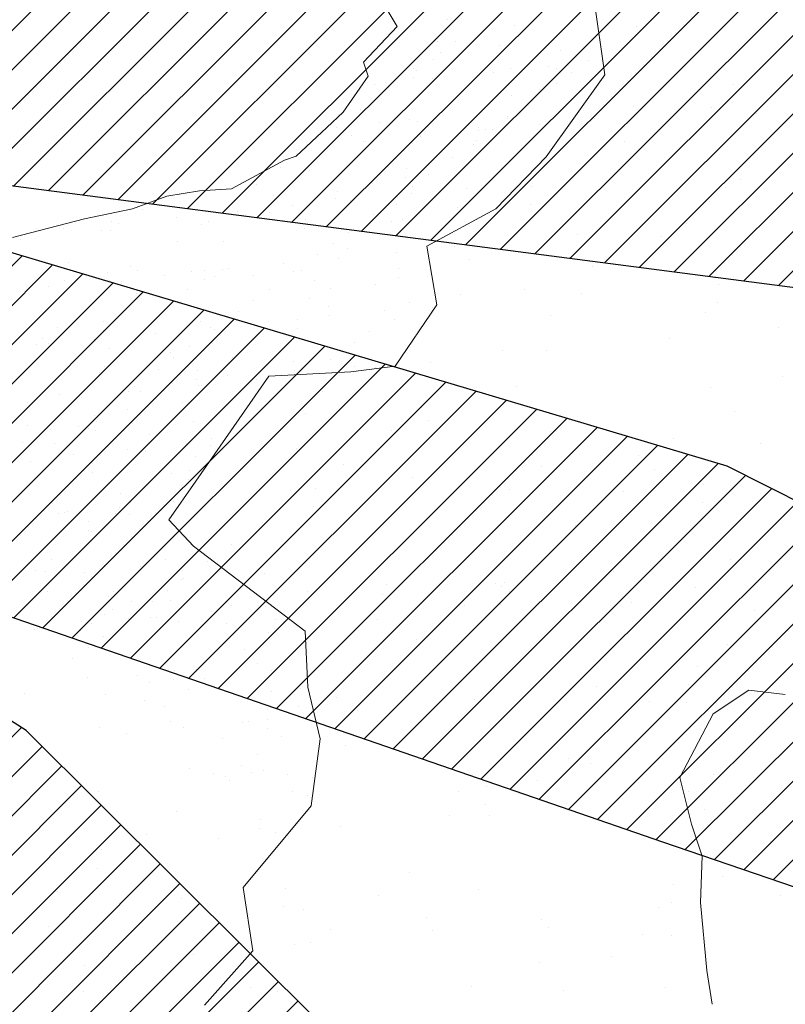
# Model space of a CAD drawing. Units: inches. Extents: x 1986 to 21484, y -1816 to 2016.
# Tile 69 of 85: x 3674.872 to 3679.11, y 1877.893 to 1883.347. Entities that reach past the tile are written whole.
import ezdxf

# ---------------------------------------------------------------- set-up
doc = ezdxf.new("R2010")
doc.units = ezdxf.units.IN
doc.layers.add('L-PLNT', color=84, linetype='Continuous', lineweight=13)
doc.layers.add('vfolhas', color=114, linetype='Continuous', lineweight=5)
for name, color, linetype in [('vfolha', 72, 'Continuous'), ('vfolha2', 110, 'Continuous'), ('vfolhas2', 102, 'Continuous')]:
    doc.layers.add(name, color=color, linetype=linetype)
pattern_1 = [(45, (-2446.5133113, 50.986076), (-0.004419417382, 0.004419417382), [])]

# ---------------------------------------------------------------- blocks, each defined once
blk = doc.blocks.new('arbusto_PB_verde_grande')
at = {"layer": 'vfolha2'}
h = blk.add_hatch(dxfattribs=at)
h.set_pattern_fill('ANSI31', color=256, scale=0.05, style=0)
h.set_pattern_definition(pattern_1)
h.paths.add_polyline_path([(0.02944, 0.35651), (0.00028, 0.09048), (0.02625, -0.03934), (0.047, 0.06233), (0.06189, 0.09731), (0.09372, 0.26573), (0.09955, 0.43473), (0.08789, 0.61313), (0.0645, 0.72266), (0.04988, 0.6851), (0.0236, 0.51294)])
h.paths.add_polyline_path([(0.30106, 0.43789), (0.14225, 0.24871), (0.26685, 0.30022)])
h.paths.add_polyline_path([(0.37995, 0.22817), (0.23697, 0.15193), (0.18428, 0.09364), (0.11122, 0.04358), (0.02625, -0.03934), (0.28061, 0.04667), (0.36829, 0.07798), (0.46756, 0.11239), (0.61068, 0.19376), (0.71585, 0.27823), (0.55813, 0.25948)])
h.paths.add_polyline_path([(0.56101, -0.29441), (0.72752, -0.32573), (0.59024, -0.2412), (0.42962, -0.15982), (0.02625, -0.03934), (0.14922, -0.14107), (0.18838, -0.16604), (0.41501, -0.24435)])
h.paths.add_polyline_path([(-0.27429, -0.44776), (-0.30352, -0.72628), (-0.23923, -0.64175), (-0.15457, -0.45716), (0.02625, -0.03934), (-0.16328, -0.25376)])
h.paths.add_polyline_path([(-0.51963, -0.24744), (-0.67736, -0.32573), (-0.59558, -0.35072), (-0.40574, -0.32882), (-0.21007, -0.20995), (0.02625, -0.03934), (-0.14874, -0.06595), (-0.31518, -0.09101), (-0.41452, -0.15048)])
h.paths.add_polyline_path([(-0.52546, 0.25007), (-0.70947, 0.24698), (-0.51963, 0.1093), (-0.32979, 0.02167), (-0.07567, -0.0128), (-0.04234, -0.02148), (-0.35024, 0.1312)])
at = {"layer": 'vfolhas'}
h = blk.add_hatch(dxfattribs=at)
h.set_pattern_fill('ANSI31', color=256, scale=0.05, style=0)
h.set_pattern_definition(pattern_1)
h.paths.add_polyline_path([(-0.07279, 0.50669), (-0.18085, 0.65063), (-0.2334, 0.67253), (-0.20712, 0.53176), (-0.10785, 0.25007), (0.02625, -0.03934), (0.00028, 0.09048), (0.00816, 0.16241), (-0.04939, 0.29079)])
h.paths.add_polyline_path([(0.09902, 0.41929), (0.09372, 0.26573), (0.07906, 0.18814), (0.15506, 0.36901), (0.26606, 0.5505), (0.28356, 0.63504), (0.2485, 0.68819), (0.25145, 0.63504), (0.20178, 0.54426)])
h.paths.add_polyline_path([(0.12295, 0.24073), (0.047, 0.06233), (0.02625, -0.03934), (0.11122, 0.04358), (0.18428, 0.09364), (0.27478, 0.19376), (0.3215, 0.25323), (0.44129, 0.38467), (0.47634, 0.57866), (0.41789, 0.45347), (0.28939, 0.30954)])
h.paths.add_polyline_path([(0.58145, -0.03779), (0.70707, 0.01536), (0.78591, 0.04667), (0.74796, 0.06549), (0.62818, 0.08423), (0.52595, 0.09048), (0.39745, 0.04358), (0.02625, -0.03934), (0.25728, -0.03154), (0.43834, -0.0347)])
h.paths.add_polyline_path([(0.52022, -0.03647), (0.43834, -0.0347), (0.25728, -0.03154), (0.02625, -0.03934), (0.17964, -0.08515), (0.53768, -0.13167), (0.69541, -0.15357), (0.78591, -0.07852), (0.70413, -0.10042)])
h.paths.add_polyline_path([(0.27189, -0.21929), (0.14922, -0.14107), (0.02625, -0.03934), (0.15794, -0.31007), (0.29522, -0.42585), (0.41789, -0.49157), (0.56396, -0.56669), (0.5114, -0.48532), (0.39456, -0.34139)])
h.paths.add_polyline_path([(-0.05818, -0.47591), (-0.02312, -0.61984), (0.047, -0.80134), (0.08494, -0.59794), (0.07911, -0.4071), (0.03527, -0.25376), (0.02625, -0.03934), (-0.03773, -0.26001)])
h.paths.add_polyline_path([(-0.24218, 0.14054), (-0.11073, 0.06858), (0.02625, -0.03934), (-0.04235, 0.10871), (-0.21007, 0.23757), (-0.36485, 0.33145), (-0.47874, 0.40341), (-0.54303, 0.46288), (-0.49041, 0.33145), (-0.39408, 0.22192)])
at = {"layer": 'vfolha'}
for p, q in [((0.53768, -0.13167), (0.17964, -0.08515)), ((0.39456, -0.34139), (0.27189, -0.21929))]:
    blk.add_line(p, q, dxfattribs=at)
at = {"layer": 'vfolha2'}
for p, q in [((0.42962, -0.15982), (0.02625, -0.03934)), ((0.59024, -0.2412), (0.42962, -0.15982)), ((0.18838, -0.16604), (0.41501, -0.24435)), ((0.41501, -0.24435), (0.56101, -0.29441))]:
    blk.add_line(p, q, dxfattribs=at)
at = {"layer": 'vfolhas2'}
blk.add_line((0.27189, -0.21929), (0.14922, -0.14107), dxfattribs=at)
blk = doc.blocks.new('PLANT-SHRUB')
for p, q in [((2160.9334, 1900.8779), (2161.0374, 1901.0337)), ((2160.3523, 1900.855), (2160.3523, 1900.855)), ((2160.6996, 1900.5794), (2160.9334, 1900.8779)), ((2161.1627, 1900.7886), (2161.1627, 1900.7886)), ((2160.1875, 1900.5998), (2160.1875, 1900.5998)), ((2160.5177, 1900.3976), (2160.6996, 1900.5794)), ((2160.6996, 1900.5794), (2160.6996, 1900.5794)), ((2160.9394, 1900.6033), (2160.9394, 1900.6033)), ((2160.5124, 1900.557), (2160.5124, 1900.557)), ((2160.815, 1900.47), (2160.815, 1900.47)), ((2161.0553, 1900.4856), (2161.0553, 1900.4856)), ((2160.8913, 1900.4413), (2160.8913, 1900.4413)), ((2161.2633, 1900.4582), (2161.2633, 1900.4582)), ((2161.5883, 1900.4154), (2161.5883, 1900.4154)), ((2160.4398, 1900.2289), (2160.5177, 1900.3976)), ((2160.7413, 1900.4025), (2160.7413, 1900.4025)), ((2160.3099, 1899.9952), (2160.4398, 1900.2289)), ((2160.3327, 1900.2167), (2160.3327, 1900.2167)), ((2161.5773, 1900.2145), (2161.5773, 1900.2145)), ((2160.1641, 1900.1094), (2160.1641, 1900.1094)), ((2160.3271, 1900.0849), (2160.3271, 1900.0849)), ((2161.4088, 1900.1071), (2161.4088, 1900.1071)), ((2159.5694, 1900.0601), (2159.6993, 1899.9044)), ((2160.3435, 1900.038), (2160.3435, 1900.038)), ((2161.4066, 1900.046), (2161.4066, 1900.046)), ((2161.9428, 1900.0517), (2161.9428, 1900.0517)), ((2159.9332, 1899.8654), (2160.3099, 1899.9952)), ((2159.6993, 1899.9044), (2159.9332, 1899.8654)), ((2159.9958, 1899.7194), (2159.9958, 1899.7194)), ((2159.82, 1899.6846), (2159.82, 1899.6846)), ((2159.9222, 1899.6519), (2159.9222, 1899.6519)), ((2160.8662, 1899.6713), (2160.8662, 1899.6713)), ((2161.545, 1899.6872), (2161.545, 1899.6872)), ((2161.8885, 1899.6762), (2161.8885, 1899.6762)), ((2159.372, 1899.6047), (2159.372, 1899.6047)), ((2159.611, 1899.6409), (2159.611, 1899.6409)), ((2159.819, 1899.6135), (2159.819, 1899.6135)), ((2160.6166, 1899.6024), (2160.6166, 1899.6024)), ((2161.8613, 1899.6002), (2161.8613, 1899.6002)), ((2160.1439, 1899.5708), (2160.1439, 1899.5708)), ((2160.6868, 1899.4993), (2160.6868, 1899.4993)), ((2160.8948, 1899.4719), (2160.8948, 1899.4719)), ((2161.2198, 1899.4291), (2161.2198, 1899.4291)), ((2161.1973, 1899.3686), (2161.1973, 1899.3686)), ((2161.7626, 1899.3576), (2161.7626, 1899.3576)), ((2161.9707, 1899.3303), (2161.9707, 1899.3303)), ((2162.7465, 1899.3364), (2162.7465, 1899.3364)), ((2159.2795, 1899.3099), (2159.2795, 1899.3099)), ((2159.5244, 1899.2874), (2159.5244, 1899.2874)), ((2160.3019, 1899.3148), (2160.3019, 1899.3148)), ((2161.1236, 1899.3011), (2161.1236, 1899.3011)), ((2161.3814, 1899.2759), (2161.3814, 1899.2759)), ((2162.2956, 1899.2875), (2162.2956, 1899.2875)), ((2160.0099, 1899.2159), (2160.0099, 1899.2159)), ((2161.2545, 1899.2136), (2161.2545, 1899.2136)), ((2162.4276, 1899.2625), (2162.4276, 1899.2625)), ((2162.4991, 1899.2114), (2162.4991, 1899.2114)), ((2162.8385, 1899.216), (2162.8385, 1899.216)), ((2159.8413, 1899.1085), (2159.8413, 1899.1085)), ((2161.086, 1899.1063), (2161.086, 1899.1063)), ((2162.3306, 1899.104), (2162.3306, 1899.104)), ((2162.6895, 1899.0787), (2163.0906, 1899.1151)), ((2162.4889, 1898.7872), (2162.6895, 1899.0787)), ((2162.3988, 1899.0178), (2162.3988, 1899.0178)), ((2158.7153, 1898.9534), (2158.7153, 1898.9534)), ((2159.1767, 1898.9688), (2159.1767, 1898.9688)), ((2160.7258, 1898.9366), (2160.7258, 1898.9366)), ((2162.3251, 1898.9503), (2162.3251, 1898.9503)), ((2159.103, 1898.9013), (2159.103, 1898.9013)), ((2159.7948, 1898.9145), (2159.7948, 1898.9145)), ((2160.841, 1898.9012), (2160.841, 1898.9012)), ((2161.8634, 1898.9061), (2161.8634, 1898.9061)), ((2162.9428, 1898.8672), (2162.9428, 1898.8672)), ((2161.9054, 1898.7143), (2162.4889, 1898.7872)), ((2162.4889, 1898.7872), (2162.4889, 1898.7872)), ((2158.3747, 1898.7689), (2158.3747, 1898.7689)), ((2158.6996, 1898.7261), (2158.6996, 1898.7261)), ((2161.6137, 1898.4774), (2161.9054, 1898.7143)), ((2162.1495, 1898.6865), (2162.1495, 1898.6865)), ((2159.2425, 1898.6546), (2159.2425, 1898.6546)), ((2159.4505, 1898.6272), (2159.4505, 1898.6272)), ((2160.3781, 1898.618), (2160.3781, 1898.618)), ((2161.877, 1898.6584), (2161.877, 1898.6584)), ((2159.0492, 1898.6039), (2159.0492, 1898.6039)), ((2159.7754, 1898.5845), (2159.7754, 1898.5845)), ((2160.2938, 1898.6016), (2160.2938, 1898.6016)), ((2161.5385, 1898.5994), (2161.5385, 1898.5994)), ((2161.7927, 1898.6047), (2161.7927, 1898.6047)), ((2161.9273, 1898.5858), (2161.9273, 1898.5858)), ((2161.9273, 1898.5858), (2161.9273, 1898.5858)), ((2162.1613, 1898.575), (2162.1613, 1898.575)), ((2162.1981, 1898.6088), (2162.1981, 1898.6088)), ((2162.7831, 1898.5971), (2162.7831, 1898.5971)), ((2163.5266, 1898.5995), (2163.5266, 1898.5995)), ((2158.2082, 1898.5531), (2158.2082, 1898.5531)), ((2158.7052, 1898.5367), (2158.7052, 1898.5367)), ((2159.2544, 1898.5398), (2159.2544, 1898.5398)), ((2160.2768, 1898.5447), (2160.2768, 1898.5447)), ((2160.3044, 1898.5505), (2160.3044, 1898.5505)), ((2160.3183, 1898.513), (2160.3183, 1898.513)), ((2161.3562, 1898.5058), (2161.3562, 1898.5058)), ((2160.5263, 1898.4856), (2160.5263, 1898.4856)), ((2161.4678, 1898.2224), (2161.6137, 1898.4774)), ((2161.6137, 1898.4774), (2161.6137, 1898.4774)), ((2161.8793, 1898.4991), (2161.8793, 1898.4991)), ((2162.4024, 1898.4924), (2162.4024, 1898.4924)), ((2163.4248, 1898.4973), (2163.4248, 1898.4973)), ((2160.8513, 1898.4428), (2160.8513, 1898.4428)), ((2161.9624, 1898.3927), (2161.9624, 1898.3927)), ((2161.3941, 1898.3714), (2161.3941, 1898.3714)), ((2161.6022, 1898.344), (2161.6022, 1898.344)), ((2161.6022, 1898.344), (2161.6022, 1898.344)), ((2161.6022, 1898.344), (2161.6022, 1898.344)), ((2162.0189, 1898.3513), (2162.0189, 1898.3513)), ((2161.5972, 1898.3209), (2161.5972, 1898.3209)), ((2161.7646, 1898.3226), (2161.7646, 1898.3226)), ((2161.9271, 1898.3012), (2161.9271, 1898.3012)), ((2161.9271, 1898.3012), (2161.9271, 1898.3012)), ((2162.0361, 1898.2868), (2162.0361, 1898.2868)), ((2162.1369, 1898.3014), (2162.1369, 1898.3014)), ((2161.5796, 1898.2672), (2161.5796, 1898.2672)), ((2161.5796, 1898.2672), (2161.5796, 1898.2672)), ((2161.7885, 1898.2334), (2161.7885, 1898.2334)), ((2162.1401, 1898.2731), (2162.1401, 1898.2731)), ((2162.47, 1898.2297), (2162.47, 1898.2297)), ((2163.1287, 1898.235), (2163.1287, 1898.235)), ((2158.3575, 1898.2181), (2158.3575, 1898.2181)), ((2158.4425, 1898.2174), (2158.4425, 1898.2174)), ((2158.6902, 1898.1833), (2158.6902, 1898.1833)), ((2159.6871, 1898.2151), (2159.6871, 1898.2151)), ((2159.9066, 1898.186), (2159.9066, 1898.186)), ((2160.9317, 1898.2128), (2160.9317, 1898.2128)), ((2161.2673, 1897.9855), (2161.4678, 1898.2224)), ((2161.5059, 1898.1997), (2161.5059, 1898.1997)), ((2161.5059, 1898.1997), (2161.5059, 1898.1997)), ((2161.7517, 1898.1997), (2161.7517, 1898.1997)), ((2162.1764, 1898.2106), (2162.1764, 1898.2106)), ((2162.1764, 1898.2106), (2162.1764, 1898.2106)), ((2162.678, 1898.2023), (2162.678, 1898.2023)), ((2163.421, 1898.2083), (2163.421, 1898.2083)), ((2158.2838, 1898.1506), (2158.2838, 1898.1506)), ((2159.7696, 1898.1444), (2159.7696, 1898.1444)), ((2160.8158, 1898.1311), (2160.8158, 1898.1311)), ((2161.7156, 1898.158), (2161.7156, 1898.158)), ((2161.8382, 1898.136), (2161.8382, 1898.136)), ((2161.8382, 1898.136), (2161.8382, 1898.136)), ((2163.0029, 1898.1596), (2163.0029, 1898.1596)), ((2158.2739, 1898.11), (2158.2739, 1898.11)), ((2159.5186, 1898.1077), (2159.5186, 1898.1077)), ((2160.7632, 1898.1055), (2160.7632, 1898.1055)), ((2161.6313, 1898.1043), (2161.6313, 1898.1043)), ((2161.8667, 1898.1141), (2161.8667, 1898.1141)), ((2162.0078, 1898.1032), (2162.0078, 1898.1032)), ((2162.0078, 1898.1032), (2162.0078, 1898.1032)), ((2162.2536, 1898.1032), (2162.2536, 1898.1032)), ((2162.9177, 1898.0971), (2162.9177, 1898.0971)), ((2163.2525, 1898.1009), (2163.2525, 1898.1009)), ((2161.5528, 1898.0174), (2161.5528, 1898.0174)), ((2161.3949, 1897.2203), (2161.2673, 1897.9855)), ((2161.5846, 1897.9358), (2161.5846, 1897.9358)), ((2162.1244, 1897.9164), (2162.1244, 1897.9164)), ((2162.781, 1897.9164), (2162.781, 1897.9164)), ((2159.5589, 1897.8673), (2159.5589, 1897.8673)), ((2161.3139, 1897.8645), (2161.3139, 1897.8645)), ((2161.379, 1897.8581), (2161.379, 1897.8581)), ((2161.4179, 1897.8508), (2161.4179, 1897.8508)), ((2161.8576, 1897.8509), (2161.8576, 1897.8509)), ((2162.7074, 1897.8489), (2162.7074, 1897.8489)), ((2157.7982, 1897.81), (2157.7982, 1897.81)), ((2159.4853, 1897.7998), (2159.4853, 1897.7998)), ((2161.1081, 1897.8352), (2161.1081, 1897.8352)), ((2161.3421, 1897.8244), (2161.3421, 1897.8244)), ((2161.5804, 1897.8294), (2161.5804, 1897.8294)), ((2161.8518, 1897.7937), (2161.8518, 1897.7937)), ((2162.1535, 1897.842), (2162.1535, 1897.842)), ((2157.886, 1897.7861), (2157.886, 1897.7861)), ((2158.0062, 1897.7826), (2158.0062, 1897.7826)), ((2158.183, 1897.783), (2158.183, 1897.783)), ((2158.3311, 1897.7398), (2158.3311, 1897.7398)), ((2159.2292, 1897.7697), (2159.2292, 1897.7697)), ((2160.2516, 1897.7746), (2160.2516, 1897.7746)), ((2161.9558, 1897.78), (2161.9558, 1897.78)), ((2162.1183, 1897.7586), (2162.1183, 1897.7586)), ((2161.3311, 1897.7357), (2161.3311, 1897.7357)), ((2161.3311, 1897.7357), (2161.3311, 1897.7357)), ((2161.3311, 1897.7357), (2161.3311, 1897.7357)), ((2161.8541, 1897.729), (2161.8541, 1897.729)), ((2161.9797, 1897.6827), (2161.9797, 1897.6827)), ((2162.3772, 1897.7223), (2162.3772, 1897.7223)), ((2158.874, 1897.6683), (2158.874, 1897.6683)), ((2159.082, 1897.6409), (2159.082, 1897.6409)), ((2161.5542, 1897.6576), (2161.5542, 1897.6576)), ((2161.9429, 1897.649), (2161.9429, 1897.649)), ((2162.1765, 1897.6565), (2162.1765, 1897.6565)), ((2157.4818, 1897.6053), (2157.4818, 1897.6053)), ((2158.7264, 1897.6031), (2158.7264, 1897.6031)), ((2159.4069, 1897.5982), (2159.4069, 1897.5982)), ((2159.9711, 1897.6008), (2159.9711, 1897.6008)), ((2161.2157, 1897.5986), (2161.2157, 1897.5986)), ((2161.4699, 1897.6039), (2161.4699, 1897.6039)), ((2162.0922, 1897.6028), (2162.0922, 1897.6028)), ((2162.4603, 1897.5963), (2162.4603, 1897.5963)), ((2159.9498, 1897.5267), (2159.9498, 1897.5267)), ((2161.572, 1897.5508), (2161.572, 1897.5508)), ((2162.1118, 1897.5313), (2162.1118, 1897.5313)), ((2157.5383, 1897.4675), (2157.5383, 1897.4675)), ((2160.1578, 1897.4993), (2160.1578, 1897.4993)), ((2160.7604, 1897.5166), (2160.7604, 1897.5166)), ((2161.7439, 1897.4667), (2161.7439, 1897.4667)), ((2162.3096, 1897.4844), (2162.3096, 1897.4844)), ((2162.3096, 1897.4844), (2162.3096, 1897.4844)), ((2158.665, 1897.4132), (2158.665, 1897.4132)), ((2159.0875, 1897.4353), (2159.0875, 1897.4353)), ((2160.4828, 1897.4565), (2160.4828, 1897.4565)), ((2160.6867, 1897.449), (2160.6867, 1897.449)), ((2157.4646, 1897.4), (2157.4646, 1897.4)), ((2157.6426, 1897.4083), (2157.6426, 1897.4083)), ((2159.7444, 1897.3743), (2159.7444, 1897.3743)), ((2160.7906, 1897.361), (2160.7906, 1897.361)), ((2161.0256, 1897.3851), (2161.0256, 1897.3851)), ((2161.2337, 1897.3577), (2161.2337, 1897.3577)), ((2161.813, 1897.3659), (2161.813, 1897.3659)), ((2161.813, 1897.3659), (2161.813, 1897.3659)), ((2161.3961, 1897.3363), (2161.3961, 1897.3363)), ((2161.5586, 1897.3149), (2161.5586, 1897.3149)), ((2161.5586, 1897.3149), (2161.5586, 1897.3149)), ((2161.5701, 1897.3074), (2161.5701, 1897.3074)), ((2161.6676, 1897.3005), (2161.6676, 1897.3005)), ((2161.6962, 1897.3505), (2161.6962, 1897.3505)), ((2161.8416, 1897.344), (2161.8416, 1897.344)), ((2162.3185, 1897.3493), (2162.3185, 1897.3493)), ((2159.4986, 1897.1656), (2159.8997, 1897.2567)), ((2159.8997, 1897.2567), (2160.1003, 1897.1109)), ((2159.8997, 1897.2567), (2159.8997, 1897.2567)), ((2161.5333, 1897.2737), (2161.5333, 1897.2737)), ((2161.7716, 1897.2869), (2161.7716, 1897.2869)), ((2161.934, 1897.2655), (2161.934, 1897.2655)), ((2158.1197, 1897.2165), (2158.1197, 1897.2165)), ((2159.3643, 1897.2143), (2159.3643, 1897.2143)), ((2160.6089, 1897.212), (2160.6089, 1897.212)), ((2161.3949, 1897.0199), (2161.3949, 1897.2203)), ((2161.8536, 1897.2098), (2161.8536, 1897.2098)), ((2161.8536, 1897.2098), (2161.8536, 1897.2098)), ((2162.1015, 1897.2434), (2162.1015, 1897.2434)), ((2162.1015, 1897.2434), (2162.1015, 1897.2434)), ((2162.2055, 1897.2297), (2162.2055, 1897.2297)), ((2162.3095, 1897.216), (2162.3095, 1897.216)), ((2162.3095, 1897.216), (2162.3095, 1897.216)), ((2162.3095, 1897.216), (2162.3095, 1897.216)), ((2159.3162, 1896.8923), (2159.4986, 1897.1656)), ((2159.5258, 1897.1606), (2159.5258, 1897.1606)), ((2159.9854, 1897.1894), (2159.9854, 1897.1894)), ((2161.5594, 1897.1657), (2161.5594, 1897.1657)), ((2161.9619, 1897.1658), (2161.9619, 1897.1658)), ((2161.9619, 1897.1658), (2161.9619, 1897.1658)), ((2162.0151, 1897.1561), (2162.0151, 1897.1561)), ((2162.0992, 1897.1463), (2162.0992, 1897.1463)), ((2162.6344, 1897.1733), (2162.6344, 1897.1733)), ((2157.9511, 1897.1092), (2157.9511, 1897.1092)), ((2158.7398, 1897.1167), (2158.7398, 1897.1167)), ((2159.1958, 1897.1069), (2159.1958, 1897.1069)), ((2160.0639, 1897.1058), (2160.0639, 1897.1058)), ((2160.1003, 1897.1109), (2160.4467, 1896.8194)), ((2160.2889, 1897.0845), (2160.2889, 1897.0845)), ((2160.4404, 1897.1046), (2160.4404, 1897.1046)), ((2161.685, 1897.1024), (2161.685, 1897.1024)), ((2161.685, 1897.1024), (2161.685, 1897.1024)), ((2161.8882, 1897.0983), (2161.8882, 1897.0983)), ((2161.8882, 1897.0983), (2161.8882, 1897.0983)), ((2161.9308, 1897.1024), (2161.9308, 1897.1024)), ((2162.134, 1897.0983), (2162.134, 1897.0983)), ((2162.1708, 1897.132), (2162.1708, 1897.132)), ((2158.6661, 1897.0492), (2158.6661, 1897.0492)), ((2159.5981, 1897.0556), (2159.5981, 1897.0556)), ((2159.7233, 1897.0669), (2159.7233, 1897.0669)), ((2157.9487, 1896.8741), (2158.4957, 1896.9834)), ((2158.1578, 1897.0129), (2158.1578, 1897.0129)), ((2158.4957, 1896.9834), (2158.8968, 1897.0016)), ((2158.4957, 1896.9834), (2158.4957, 1896.9834)), ((2158.8968, 1897.0016), (2159.3162, 1896.8923)), ((2158.8968, 1897.0016), (2158.8968, 1897.0016)), ((2159.204, 1896.9996), (2159.204, 1896.9996)), ((2159.7319, 1896.9893), (2159.7319, 1896.9893)), ((2159.8696, 1897.0198), (2159.8696, 1897.0198)), ((2159.9736, 1897.0062), (2159.9736, 1897.0062)), ((2160.1361, 1896.9848), (2160.1361, 1896.9848)), ((2160.2264, 1897.0045), (2160.2264, 1897.0045)), ((2160.2264, 1897.0045), (2160.2264, 1897.0045)), ((2161.1396, 1896.9652), (2161.3949, 1897.0199)), ((2160.4467, 1896.8194), (2161.1396, 1896.9652)), ((2161.1605, 1896.9321), (2161.1605, 1896.9321)), ((2161.3059, 1896.9656), (2161.3059, 1896.9656)), ((2161.3059, 1896.9656), (2161.3059, 1896.9656)), ((2161.3059, 1896.9656), (2161.3059, 1896.9656)), ((2161.829, 1896.9589), (2161.829, 1896.9589)), ((2162.3402, 1896.9614), (2162.3402, 1896.9614)), ((2162.3521, 1896.9523), (2162.3521, 1896.9523)), ((2162.3521, 1896.9523), (2162.3521, 1896.9523)), ((2157.6934, 1896.5097), (2157.9487, 1896.8741)), ((2158.713, 1896.8669), (2158.713, 1896.8669)), ((2159.5126, 1896.8738), (2159.5126, 1896.8738)), ((2159.5495, 1896.9076), (2159.5495, 1896.9076)), ((2160.324, 1896.8915), (2160.324, 1896.8915)), ((2160.9454, 1896.8782), (2160.9454, 1896.8782)), ((2161.0494, 1896.8645), (2161.0494, 1896.8645)), ((2161.1237, 1896.8983), (2161.1237, 1896.8983)), ((2161.9351, 1896.916), (2161.9351, 1896.916)), ((2158.3988, 1896.828), (2158.3988, 1896.828)), ((2158.4232, 1896.8557), (2158.4232, 1896.8557)), ((2159.0455, 1896.8546), (2159.0455, 1896.8546)), ((2159.6678, 1896.8534), (2159.6678, 1896.8534)), ((2160.2901, 1896.8523), (2160.2901, 1896.8523)), ((2160.4467, 1896.8194), (2160.4467, 1896.8194)), ((2160.9125, 1896.8512), (2160.9125, 1896.8512)), ((2161.2119, 1896.8431), (2161.2119, 1896.8431)), ((2161.5348, 1896.8501), (2161.5348, 1896.8501)), ((2162.1571, 1896.8489), (2162.1571, 1896.8489)), ((2157.6377, 1896.7963), (2157.6377, 1896.7963)), ((2158.9386, 1896.8086), (2158.9386, 1896.8086)), ((2159.4616, 1896.8019), (2159.4616, 1896.8019)), ((2159.9412, 1896.7659), (2159.9412, 1896.7659)), ((2159.9412, 1896.7659), (2159.9412, 1896.7659)), ((2159.9728, 1896.8044), (2159.9728, 1896.8044)), ((2160.5126, 1896.7849), (2160.5126, 1896.7849)), ((2161.0357, 1896.7782), (2161.0357, 1896.7782)), ((2161.4833, 1896.8074), (2161.4833, 1896.8074)), ((2161.5469, 1896.7807), (2161.5469, 1896.7807)), ((2161.5873, 1896.7937), (2161.5873, 1896.7937)), ((2161.7498, 1896.7723), (2161.7498, 1896.7723)), ((2161.7612, 1896.7567), (2161.7612, 1896.7567)), ((2162.0866, 1896.7612), (2162.0866, 1896.7612)), ((2157.9626, 1896.7535), (2157.9626, 1896.7535)), ((2157.9626, 1896.7535), (2157.9626, 1896.7535)), ((2158.0716, 1896.7392), (2158.0716, 1896.7392)), ((2158.1756, 1896.7255), (2158.1756, 1896.7255)), ((2158.3381, 1896.7041), (2158.3381, 1896.7041)), ((2158.5391, 1896.7076), (2158.5391, 1896.7076)), ((2160.1502, 1896.7322), (2160.1502, 1896.7322)), ((2160.9248, 1896.7161), (2160.9248, 1896.7161)), ((2161.4904, 1896.7337), (2161.4904, 1896.7337)), ((2161.4904, 1896.7337), (2161.4904, 1896.7337)), ((2161.7244, 1896.7229), (2161.7244, 1896.7229)), ((2162.0212, 1896.7366), (2162.0212, 1896.7366)), ((2162.1252, 1896.7229), (2162.1252, 1896.7229)), ((2158.1198, 1896.6624), (2158.1198, 1896.6624)), ((2158.2683, 1896.6847), (2158.2683, 1896.6847)), ((2158.2683, 1896.6847), (2158.2683, 1896.6847)), ((2158.5023, 1896.6739), (2158.5023, 1896.6739)), ((2158.5055, 1896.682), (2158.5055, 1896.682)), ((2158.5055, 1896.682), (2158.5055, 1896.682)), ((2158.6095, 1896.6683), (2158.6095, 1896.6683)), ((2158.7135, 1896.6546), (2158.7135, 1896.6546)), ((2158.7135, 1896.6546), (2158.7135, 1896.6546)), ((2158.7135, 1896.6546), (2158.7135, 1896.6546)), ((2158.7421, 1896.6613), (2158.7421, 1896.6613)), ((2159.3137, 1896.6915), (2159.3137, 1896.6915)), ((2159.3644, 1896.6602), (2159.3644, 1896.6602)), ((2159.8676, 1896.6984), (2159.8676, 1896.6984)), ((2159.8676, 1896.6984), (2159.8676, 1896.6984)), ((2159.9868, 1896.659), (2159.9868, 1896.659)), ((2160.1134, 1896.6984), (2160.1134, 1896.6984)), ((2160.6091, 1896.6579), (2160.6091, 1896.6579)), ((2161.2314, 1896.6568), (2161.2314, 1896.6568)), ((2161.8537, 1896.6557), (2161.8537, 1896.6557)), ((2158.0355, 1896.6088), (2158.0355, 1896.6088)), ((2158.1453, 1896.6279), (2158.1453, 1896.6279)), ((2158.4036, 1896.6023), (2158.4036, 1896.6023)), ((2158.4036, 1896.6023), (2158.4036, 1896.6023)), ((2158.6398, 1896.6431), (2158.6398, 1896.6431)), ((2158.6398, 1896.6431), (2158.6398, 1896.6431)), ((2158.6579, 1896.6076), (2158.6579, 1896.6076)), ((2158.6683, 1896.6212), (2158.6683, 1896.6212)), ((2158.876, 1896.6333), (2158.876, 1896.6333)), ((2159.0385, 1896.6119), (2159.0385, 1896.6119)), ((2159.0385, 1896.6119), (2159.0385, 1896.6119)), ((2159.1474, 1896.5975), (2159.1474, 1896.5975)), ((2159.1795, 1896.6237), (2159.1795, 1896.6237)), ((2159.2802, 1896.6065), (2159.2802, 1896.6065)), ((2159.6483, 1896.6), (2159.6483, 1896.6)), ((2159.6483, 1896.6), (2159.6483, 1896.6)), ((2159.7193, 1896.6042), (2159.7193, 1896.6042)), ((2159.7193, 1896.6042), (2159.7193, 1896.6042)), ((2159.7193, 1896.6042), (2159.7193, 1896.6042)), ((2159.9025, 1896.6054), (2159.9025, 1896.6054)), ((2160.2424, 1896.5975), (2160.2424, 1896.5975)), ((2160.5248, 1896.6042), (2160.5248, 1896.6042)), ((2160.7536, 1896.6), (2160.7536, 1896.6)), ((2160.8929, 1896.5977), (2160.8929, 1896.5977)), ((2160.8929, 1896.5977), (2160.8929, 1896.5977)), ((2161.1471, 1896.6031), (2161.1471, 1896.6031)), ((2161.7694, 1896.602), (2161.7694, 1896.602)), ((2161.7878, 1896.5958), (2161.7878, 1896.5958)), ((2161.7878, 1896.5958), (2161.7878, 1896.5958)), ((2159.2514, 1896.5838), (2159.2514, 1896.5838)), ((2159.4139, 1896.5624), (2159.4139, 1896.5624)), ((2159.5813, 1896.5404), (2159.5813, 1896.5404)), ((2159.5813, 1896.5404), (2159.5813, 1896.5404)), ((2160.7509, 1896.5568), (2160.7509, 1896.5568)), ((2160.7654, 1896.5909), (2160.7654, 1896.5909)), ((2160.7654, 1896.5909), (2160.7654, 1896.5909)), ((2161.2933, 1896.5805), (2161.2933, 1896.5805)), ((2161.5255, 1896.5407), (2161.5255, 1896.5407)), ((2161.8164, 1896.5739), (2161.8164, 1896.5739)), ((2158.3034, 1896.4916), (2158.3034, 1896.4916)), ((2159.103, 1896.4985), (2159.103, 1896.4985)), ((2159.1399, 1896.5322), (2159.1399, 1896.5322)), ((2159.6853, 1896.5267), (2159.6853, 1896.5267)), ((2159.7894, 1896.513), (2159.7894, 1896.513)), ((2159.7894, 1896.513), (2159.7894, 1896.513)), ((2159.7894, 1896.513), (2159.7894, 1896.513)), ((2159.9145, 1896.5162), (2159.9145, 1896.5162)), ((2159.9518, 1896.4916), (2159.9518, 1896.4916)), ((2160.7141, 1896.523), (2160.7141, 1896.523)), ((2158.3862, 1896.443), (2158.3862, 1896.443)), ((2160.1143, 1896.4702), (2160.1143, 1896.4702)), ((2160.1143, 1896.4702), (2160.1143, 1896.4702)), ((2160.2232, 1896.4559), (2160.2232, 1896.4559)), ((2160.3273, 1896.4422), (2160.3273, 1896.4422)), ((2158.926, 1896.4235), (2158.926, 1896.4235)), ((2159.4491, 1896.4169), (2159.4491, 1896.4169)), ((2159.9603, 1896.4193), (2159.9603, 1896.4193)), ((2160.4897, 1896.4208), (2160.4897, 1896.4208)), ((2160.5, 1896.3999), (2160.5, 1896.3999)), ((2160.6571, 1896.3988), (2160.6571, 1896.3988)), ((2160.6571, 1896.3988), (2160.6571, 1896.3988)), ((2160.7612, 1896.3851), (2160.7612, 1896.3851)), ((2161.0231, 1896.3932), (2161.0231, 1896.3932)), ((2161.1427, 1896.4151), (2161.1427, 1896.4151)), ((2161.1427, 1896.4151), (2161.1427, 1896.4151)), ((2161.3516, 1896.3814), (2161.3516, 1896.3814)), ((2161.5343, 1896.3956), (2161.5343, 1896.3956)), ((2158.1295, 1896.3323), (2158.1295, 1896.3323)), ((2158.2618, 1896.3553), (2158.2618, 1896.3553)), ((2158.8841, 1896.3542), (2158.8841, 1896.3542)), ((2159.4698, 1896.3339), (2159.4698, 1896.3339)), ((2159.4698, 1896.3339), (2159.4698, 1896.3339)), ((2159.5064, 1896.353), (2159.5064, 1896.353)), ((2159.7038, 1896.3231), (2159.7038, 1896.3231)), ((2159.7406, 1896.3568), (2159.7406, 1896.3568)), ((2160.1287, 1896.3519), (2160.1287, 1896.3519)), ((2160.5152, 1896.3408), (2160.5152, 1896.3408)), ((2160.7511, 1896.3508), (2160.7511, 1896.3508)), ((2160.8652, 1896.3714), (2160.8652, 1896.3714)), ((2160.8652, 1896.3714), (2160.8652, 1896.3714)), ((2160.8652, 1896.3714), (2160.8652, 1896.3714)), ((2161.0276, 1896.35), (2161.0276, 1896.35)), ((2161.069, 1896.3476), (2161.069, 1896.3476)), ((2161.069, 1896.3476), (2161.069, 1896.3476)), ((2161.1901, 1896.3286), (2161.1901, 1896.3286)), ((2161.1901, 1896.3286), (2161.1901, 1896.3286)), ((2161.3148, 1896.3476), (2161.3148, 1896.3476)), ((2161.3734, 1896.3496), (2161.3734, 1896.3496)), ((2158.9041, 1896.3162), (2158.9041, 1896.3162)), ((2161.2991, 1896.3142), (2161.2991, 1896.3142)), ((2161.4031, 1896.3006), (2161.4031, 1896.3006)), ((2161.5655, 1896.2792), (2161.5655, 1896.2792)), ((2158.6558, 1896.2362), (2158.6558, 1896.2362)), ((2159.0415, 1896.2135), (2159.0415, 1896.2135)), ((2159.0415, 1896.2135), (2159.0415, 1896.2135)), ((2159.1669, 1896.2386), (2159.1669, 1896.2386)), ((2159.1788, 1896.2295), (2159.1788, 1896.2295)), ((2159.1788, 1896.2295), (2159.1788, 1896.2295)), ((2159.7067, 1896.2192), (2159.7067, 1896.2192)), ((2160.2012, 1896.2344), (2160.2012, 1896.2344)), ((2160.2012, 1896.2344), (2160.2012, 1896.2344)), ((2160.2298, 1896.2125), (2160.2298, 1896.2125)), ((2160.2862, 1896.2112), (2160.2862, 1896.2112)), ((2160.2862, 1896.2112), (2160.2862, 1896.2112)), ((2160.741, 1896.2149), (2160.741, 1896.2149)), ((2161.733, 1896.2571), (2161.733, 1896.2571)), ((2161.733, 1896.2571), (2161.733, 1896.2571)), ((2158.4253, 1896.1752), (2158.4253, 1896.1752)), ((2158.5293, 1896.1615), (2158.5293, 1896.1615)), ((2158.5807, 1896.1609), (2158.5807, 1896.1609)), ((2158.7303, 1896.1569), (2158.7303, 1896.1569)), ((2159.2031, 1896.1598), (2159.2031, 1896.1598)), ((2159.8254, 1896.1586), (2159.8254, 1896.1586)), ((2160.3413, 1896.1815), (2160.3413, 1896.1815)), ((2160.4477, 1896.1575), (2160.4477, 1896.1575)), ((2161.07, 1896.1564), (2161.07, 1896.1564)), ((2161.1159, 1896.1654), (2161.1159, 1896.1654)), ((2161.2807, 1896.1955), (2161.2807, 1896.1955)), ((2161.2807, 1896.1955), (2161.2807, 1896.1955)), ((2161.2807, 1896.1955), (2161.2807, 1896.1955)), ((2161.5308, 1896.2089), (2161.5308, 1896.2089)), ((2161.5308, 1896.2089), (2161.5308, 1896.2089)), ((2161.6923, 1896.1552), (2161.6923, 1896.1552)), ((2158.4965, 1896.1072), (2158.4965, 1896.1072)), ((2158.6917, 1896.1401), (2158.6917, 1896.1401)), ((2158.6934, 1896.1232), (2158.6934, 1896.1232)), ((2158.873, 1896.1061), (2158.873, 1896.1061)), ((2158.873, 1896.1061), (2158.873, 1896.1061)), ((2158.9632, 1896.1044), (2158.9632, 1896.1044)), ((2159.1188, 1896.1061), (2159.1188, 1896.1061)), ((2159.5049, 1896.1408), (2159.5049, 1896.1408)), ((2159.7411, 1896.105), (2159.7411, 1896.105)), ((2160.1176, 1896.1038), (2160.1176, 1896.1038)), ((2160.1176, 1896.1038), (2160.1176, 1896.1038)), ((2160.3045, 1896.1477), (2160.3045, 1896.1477)), ((2160.3634, 1896.1038), (2160.3634, 1896.1038)), ((2160.9857, 1896.1027), (2160.9857, 1896.1027)), ((2161.3623, 1896.1016), (2161.3623, 1896.1016)), ((2161.3623, 1896.1016), (2161.3623, 1896.1016)), ((2161.6081, 1896.1016), (2161.6081, 1896.1016)), ((2158.3736, 1896.0579), (2158.3736, 1896.0579)), ((2159.0672, 1896.0907), (2159.0672, 1896.0907)), ((2159.2297, 1896.0693), (2159.2297, 1896.0693)), ((2158.9085, 1895.9822), (2159.1461, 1896.0331)), ((2158.9134, 1896.0385), (2158.9134, 1896.0385)), ((2159.1461, 1896.0331), (2159.2706, 1896.0331)), ((2159.2706, 1896.0331), (2159.5025, 1896.0331)), ((2159.5011, 1896.0336), (2159.5011, 1896.0336)), ((2159.5025, 1896.0331), (2159.5647, 1896.0048)), ((2159.5647, 1896.0048), (2159.8872, 1895.92)), ((2159.6051, 1896.0199), (2159.6051, 1896.0199)), ((2159.7676, 1895.9985), (2159.7676, 1895.9985)), ((2159.9477, 1896.0343), (2159.9477, 1896.0343)), ((2160.4874, 1896.0148), (2160.4874, 1896.0148)), ((2160.9421, 1896.0061), (2160.9421, 1896.0061)), ((2161.0105, 1896.0081), (2161.0105, 1896.0081)), ((2161.5217, 1896.0106), (2161.5217, 1896.0106)), ((2158.8746, 1895.9087), (2158.9085, 1895.9822)), ((2160.039, 1895.9627), (2160.039, 1895.9627)), ((2160.1056, 1895.9654), (2160.1056, 1895.9654)), ((2160.143, 1895.949), (2160.143, 1895.949)), ((2160.6712, 1895.9831), (2160.6712, 1895.9831)), ((2160.6712, 1895.9831), (2160.6712, 1895.9831)), ((2160.9052, 1895.9723), (2160.9052, 1895.9723)), ((2158.5295, 1895.5526), (2158.6031, 1895.8917)), ((2158.6031, 1895.8917), (2158.8746, 1895.9087)), ((2159.8872, 1895.92), (2160.023, 1895.8069)), ((2160.3055, 1895.9277), (2160.3055, 1895.9277)), ((2160.5769, 1895.8919), (2160.5769, 1895.8919)), ((2160.5897, 1895.8504), (2160.5897, 1895.8504)), ((2160.6809, 1895.8782), (2160.6809, 1895.8782)), ((2160.7284, 1895.8299), (2160.7284, 1895.8299)), ((2160.8434, 1895.8568), (2160.8434, 1895.8568)), ((2161.212, 1895.8492), (2161.212, 1895.8492)), ((2160.023, 1895.8069), (2160.1757, 1895.7052)), ((2160.2172, 1895.8274), (2160.2172, 1895.8274)), ((2160.7063, 1895.7901), (2160.7063, 1895.7901)), ((2160.7403, 1895.8208), (2160.7403, 1895.8208)), ((2160.7403, 1895.8208), (2160.7403, 1895.8208)), ((2161.1148, 1895.8211), (2161.1148, 1895.8211)), ((2161.2188, 1895.8074), (2161.2188, 1895.8074)), ((2161.2681, 1895.8105), (2161.2681, 1895.8105)), ((2160.1757, 1895.7052), (2160.3624, 1895.6261)), ((2160.3235, 1895.6645), (2160.3235, 1895.6645)), ((2160.3235, 1895.6645), (2160.3235, 1895.6645)), ((2160.3624, 1895.6261), (2160.5943, 1895.4848)), ((2160.4748, 1895.6298), (2160.4748, 1895.6298)), ((2160.5325, 1895.6307), (2160.5325, 1895.6307)), ((2160.9086, 1895.656), (2160.9086, 1895.656)), ((2160.9979, 1895.6231), (2160.9979, 1895.6231)), ((2160.4956, 1895.597), (2160.4956, 1895.597)), ((2160.5701, 1895.5969), (2160.5701, 1895.5969)), ((2160.5701, 1895.5969), (2160.5701, 1895.5969)), ((2160.8243, 1895.6023), (2160.8243, 1895.6023)), ((2160.5943, 1895.4848), (2160.9564, 1895.2869)), ((2160.5943, 1895.4848), (2160.5943, 1895.4848)), ((2160.7158, 1895.4449), (2160.7158, 1895.4449)), ((2160.8216, 1895.3423), (2160.8216, 1895.3423)), ((2160.9306, 1895.328), (2160.9306, 1895.328))]:
    blk.add_line(p, q)

msp = doc.modelspace()

# ---------------------------------------------------------------- block references
at = {"layer": 'L-PLNT', "rotation": 223.1883365522388}
msp.add_blockref('PLANT-SHRUB', (3953.27, 4742.9646), dxfattribs=at)
at = {"layer": 'L-PLNT', "xscale": 24.60366729364114, "yscale": 24.60366729364114, "zscale": 24.60366729364114}
msp.add_blockref('arbusto_PB_verde_grande', (3668.2184, 1884.8051), dxfattribs=at)

doc.saveas('drawing.dxf')
